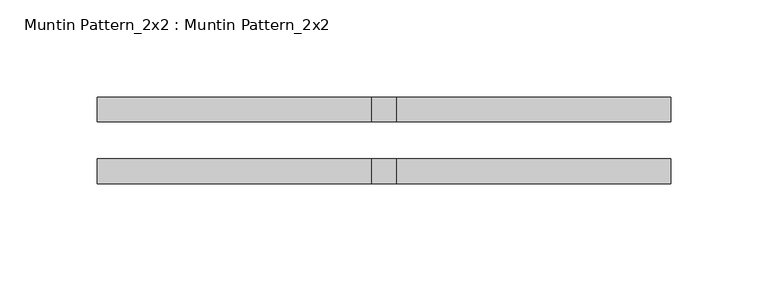
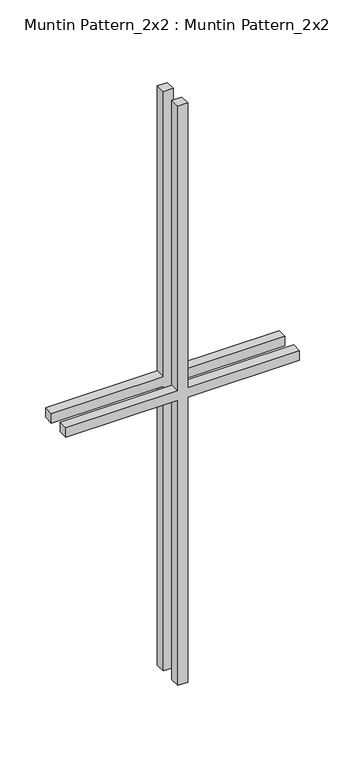
"""IFC4 building model written with IfcOpenShell, lengths in millimetres: proxy geometry, Muntin Pattern_2x2 : Muntin Pattern_2x2."""

from ifc_helpers import new_model, si_unit, frame, origin, place, context, project, spatial, polyline, outline, extrude, source, transform, mapped, element, save


def muntin_pattern_2x2_muntin_pattern_2x2_b3fe6957(model_context):
    return source(origin(), model_context, "Body", "SweptSolid", [
        extrude(outline(polyline([(393.7, -6.35), (393.7, -147.6375), (381.0, -147.6375), (381.0, -6.35), (0.0, -6.35), (0.0, 6.35), (381.0, 6.35), (381.0, 147.6375), (393.7, 147.6375), (393.7, 6.35), (774.7, 6.35), (774.7, -6.35), (393.7, -6.35)])), frame((0.0, 9.525, 0.0), z_axis=(0.0, 1.0, 0.0), x_axis=(0.0, 0.0, 1.0)), (0.0, 0.0, 1.0), 12.7),
        extrude(outline(polyline([(393.7, -6.35), (393.7, -147.6375), (381.0, -147.6375), (381.0, -6.35), (0.0, -6.35), (0.0, 6.35), (381.0, 6.35), (381.0, 147.6375), (393.7, 147.6375), (393.7, 6.35), (774.7, 6.35), (774.7, -6.35), (393.7, -6.35)])), frame((0.0, -22.225, 0.0), z_axis=(0.0, 1.0, 0.0), x_axis=(0.0, 0.0, 1.0)), (0.0, 0.0, 1.0), 12.7),
    ])


if __name__ == "__main__":
    model = new_model("IFC4")
    model_context = context("Model", 3, world=origin())
    ifc_project = project(units=[si_unit("LENGTHUNIT", "METRE", prefix="MILLI")], contexts=[model_context])
    site = spatial("IfcSite", under=ifc_project)
    building = spatial("IfcBuilding", under=site)
    placement = place(None, origin())
    muntin_pattern_2x2_muntin_pattern_2x2_shape = muntin_pattern_2x2_muntin_pattern_2x2_b3fe6957(model_context)
    element("IfcBuildingElementProxy", 1, Name="Muntin Pattern_2x2 : Muntin Pattern_2x2", ObjectType="Muntin Pattern_2x2 : Muntin Pattern_2x2", at=placement, inside=building, context=model_context, shape_type="MappedRepresentation", body=[
        mapped(muntin_pattern_2x2_muntin_pattern_2x2_shape, transform((0.0, 0.0, 0.0), x_axis=(1.0, 0.0, 0.0), y_axis=(0.0, 1.0, 0.0), z_axis=(0.0, 0.0, 1.0))),
    ])
    save(model, "model.ifc")

# Revit data of these elements
# Type "Muntin Pattern_2x2 : Muntin Pattern_2x2"
#   Width [instance default] = 4' - 0"
#   Thickness = 0' - 0 1/2"
#   Height [instance default] = 4' - 0"
#   Distance = 0' - 0 3/4"
#   Interior Material [instance default] = none
#   Exterior Material [instance default] = none
#   Default Elevation = 0
# Element 1 (IfcBuildingElementProxy, "Muntin Pattern_2x2 : Muntin Pattern_2x2")
#   Width = 0' - 11 5/8"
#   Height = 2' - 6 1/2"
#   Interior Material = Wood - Stained
#   Exterior Material = Clad - White
#   Materials on its faces: "Clad - White", "Wood - Stained"
# Materials
#   "Clad - White": class "Wood", colour RGB 30 30 30, transparency 0, Cost = 0
#   "Wood - Stained": class "Wood", colour RGB 224 178 126, transparency 0, Cost = 0
